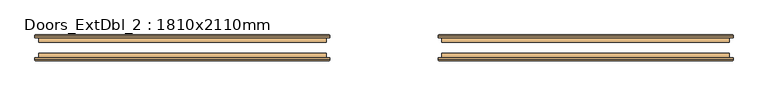
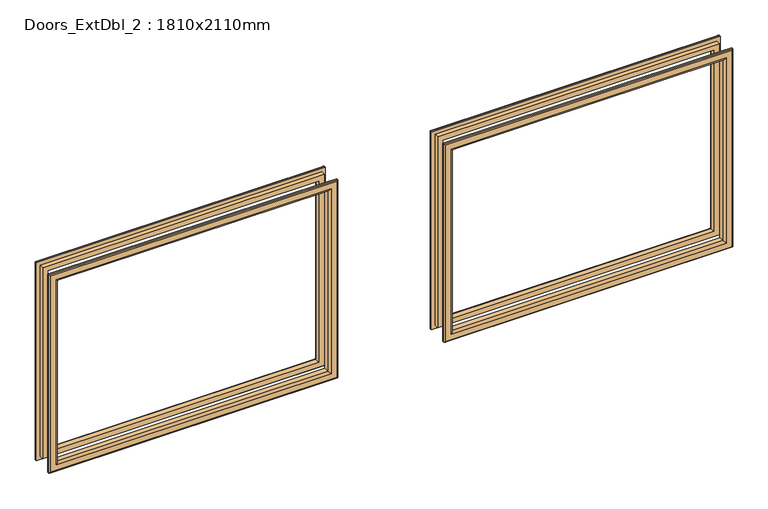
"""IFC4 building model written with IfcOpenShell, lengths in millimetres: door geometry, Doors_ExtDbl_2 : 1810x2110mm."""

from ifc_helpers import new_model, si_unit, frame, origin, place, context, project, spatial, ellipse_curve, source, transform, mapped, element, save
from ifc_brep_helpers import plane_surface, cylinder_surface, advanced_brep


def doors_extdbl_2_1810x2110mm_b7024f51(model_context):
    return source(origin(), model_context, "Body", "AdvancedBrep", [
        advanced_brep(
        [(126.5, 18.4, 808.5), (126.5, 18.4, 358.5), (126.5, 8.4, 358.5), (126.5, 8.4, 808.5), (138.5, 7.4, 796.5), (138.5, 7.4, 370.5), (138.5, 18.4, 370.5), (138.5, 18.4, 796.5), (133.5, 2.4, 801.5), (133.5, 2.4, 365.5), (118.5, 4.4, 816.5), (118.5, 4.4, 350.5), (120.5, 2.4, 352.5), (120.5, 2.4, 814.5), (118.5, 8.4, 816.5), (118.5, 8.4, 350.5), (753.5, 18.4, 358.5), (753.5, 8.4, 358.5), (741.5, 7.4, 370.5), (741.5, 18.4, 370.5), (746.5, 2.4, 365.5), (761.5, 4.4, 350.5), (759.5, 2.4, 352.5), (761.5, 8.4, 350.5), (753.5, 18.4, 808.5), (753.5, 8.4, 808.5), (741.5, 7.4, 796.5), (741.5, 18.4, 796.5), (746.5, 2.4, 801.5), (761.5, 4.4, 816.5), (759.5, 2.4, 814.5), (761.5, 8.4, 816.5)],
        [
            (0, 1),
            (1, 2),
            (2, 3),
            (3, 0),
            (4, 5),
            (5, 6),
            (6, 7),
            (7, 4),
            (8, 9),
            (9, 5, ellipse_curve(frame((133.5, 7.4, 365.5), z_axis=(-0.7071067811865475, 0.0, 0.7071067811865475), x_axis=(0.7071067811865474, 0.0, 0.7071067811865476)), 7.0710678, 5.0)),
            (4, 8, ellipse_curve(frame((133.5, 7.4, 801.5), z_axis=(-0.7071067811865475, 0.0, -0.7071067811865475), x_axis=(-0.7071067811865474, 0.0, 0.7071067811865476)), 7.0710678, 5.0)),
            (10, 11),
            (11, 12, ellipse_curve(frame((120.5, 4.4, 352.5), z_axis=(-0.7071067811865475, 0.0, 0.7071067811865475), x_axis=(0.7071067811865474, 0.0, 0.7071067811865476)), 2.8284271, 2.0)),
            (12, 13),
            (13, 10, ellipse_curve(frame((120.5, 4.4, 814.5), z_axis=(-0.7071067811865475, 0.0, -0.7071067811865475), x_axis=(-0.7071067811865474, 0.0, 0.7071067811865476)), 2.8284271, 2.0)),
            (14, 15),
            (15, 11),
            (10, 14),
            (1, 16),
            (16, 17),
            (17, 2),
            (5, 18),
            (18, 19),
            (19, 6),
            (9, 20),
            (20, 18, ellipse_curve(frame((746.5, 7.4, 365.5), z_axis=(-0.7071067811865475, 0.0, -0.7071067811865475), x_axis=(-0.7071067811865476, 0.0, 0.7071067811865474)), 7.0710678, 5.0)),
            (11, 21),
            (21, 22, ellipse_curve(frame((759.5, 4.4, 352.5), z_axis=(-0.7071067811865475, 0.0, -0.7071067811865475), x_axis=(-0.7071067811865476, 0.0, 0.7071067811865474)), 2.8284271, 2.0)),
            (22, 12),
            (15, 23),
            (23, 21),
            (16, 24),
            (24, 25),
            (25, 17),
            (18, 26),
            (26, 27),
            (27, 19),
            (20, 28),
            (28, 26, ellipse_curve(frame((746.5, 7.4, 801.5), z_axis=(0.7071067811865475, 0.0, -0.7071067811865475), x_axis=(-0.7071067811865474, 0.0, -0.7071067811865476)), 7.0710678, 5.0)),
            (21, 29),
            (29, 30, ellipse_curve(frame((759.5, 4.4, 814.5), z_axis=(0.7071067811865475, 0.0, -0.7071067811865475), x_axis=(-0.7071067811865474, 0.0, -0.7071067811865476)), 2.8284271, 2.0)),
            (30, 22),
            (23, 31),
            (31, 29),
            (14, 31),
            (25, 3),
            (24, 0),
            (27, 7),
            (26, 4),
            (28, 8),
            (30, 13),
            (29, 10),
        ],
        [
            plane_surface(frame((126.5, 8.4, 808.5), z_axis=(-1.0, 0.0, 0.0), x_axis=(0.0, 0.0, -1.0))),
            plane_surface(frame((138.5, 18.4, 796.5), z_axis=(1.0, 0.0, 0.0), x_axis=(0.0, 0.0, -1.0))),
            cylinder_surface(frame((133.5, 7.4, 808.5), z_axis=(0.0, 0.0, 1.0), x_axis=(-1.0, 0.0, 0.0)), 5.0),
            cylinder_surface(frame((120.5, 4.4, 808.5), z_axis=(0.0, 0.0, 1.0), x_axis=(-1.0, 0.0, 0.0)), 2.0),
            plane_surface(frame((118.5, 4.4, 816.5), z_axis=(-1.0, 0.0, 0.0), x_axis=(0.0, 0.0, -1.0))),
            plane_surface(frame((126.5, 8.4, 358.5), z_axis=(0.0, 0.0, -1.0), x_axis=(1.0, 0.0, 0.0))),
            plane_surface(frame((138.5, 18.4, 370.5), z_axis=(0.0, 0.0, 1.0), x_axis=(1.0, 0.0, 0.0))),
            cylinder_surface(frame((126.5, 7.4, 365.5), z_axis=(-1.0, 0.0, 0.0), x_axis=(0.0, 0.0, -1.0)), 5.0),
            cylinder_surface(frame((126.5, 4.4, 352.5), z_axis=(-1.0, 0.0, 0.0), x_axis=(0.0, 0.0, -1.0)), 2.0),
            plane_surface(frame((118.5, 4.4, 350.5), z_axis=(0.0, 0.0, -1.0), x_axis=(1.0, 0.0, 0.0))),
            plane_surface(frame((753.5, 8.4, 358.5), z_axis=(1.0, 0.0, 0.0), x_axis=(0.0, 0.0, 1.0))),
            plane_surface(frame((741.5, 18.4, 370.5), z_axis=(-1.0, 0.0, 0.0), x_axis=(0.0, 0.0, 1.0))),
            cylinder_surface(frame((746.5, 7.4, 358.5), z_axis=(0.0, 0.0, -1.0), x_axis=(1.0, 0.0, 0.0)), 5.0),
            cylinder_surface(frame((759.5, 4.4, 358.5), z_axis=(0.0, 0.0, -1.0), x_axis=(1.0, 0.0, 0.0)), 2.0),
            plane_surface(frame((761.5, 4.4, 350.5), z_axis=(1.0, 0.0, 0.0), x_axis=(0.0, 0.0, 1.0))),
            plane_surface(frame((761.5, 8.4, 816.5), z_axis=(0.0, 1.0, 0.0), x_axis=(-1.0, 0.0, 0.0))),
            plane_surface(frame((753.5, 8.4, 808.5), z_axis=(0.0, 0.0, 1.0), x_axis=(-1.0, 0.0, 0.0))),
            plane_surface(frame((753.5, 18.4, 808.5), z_axis=(0.0, 1.0, 0.0), x_axis=(-1.0, 0.0, 0.0))),
            plane_surface(frame((741.5, 18.4, 796.5), z_axis=(0.0, 0.0, -1.0), x_axis=(-1.0, 0.0, 0.0))),
            cylinder_surface(frame((753.5, 7.4, 801.5), z_axis=(1.0, 0.0, 0.0), x_axis=(0.0, 0.0, 1.0)), 5.0),
            plane_surface(frame((746.5, 2.4, 801.5), z_axis=(0.0, -1.0, 0.0), x_axis=(-1.0, 0.0, 0.0))),
            cylinder_surface(frame((753.5, 4.4, 814.5), z_axis=(1.0, 0.0, 0.0), x_axis=(0.0, 0.0, 1.0)), 2.0),
            plane_surface(frame((761.5, 4.4, 816.5), z_axis=(0.0, 0.0, 1.0), x_axis=(-1.0, 0.0, 0.0))),
        ],
        [
            (0, [[1, 2, 3, 4]]),
            (1, [[5, 6, 7, 8]]),
            (2, [[9, 10, -5, 11]]),
            (3, [[12, 13, 14, 15]]),
            (4, [[16, 17, -12, 18]]),
            (5, [[19, 20, 21, -2]]),
            (6, [[22, 23, 24, -6]]),
            (7, [[25, 26, -22, -10]]),
            (8, [[27, 28, 29, -13]]),
            (9, [[30, 31, -27, -17]]),
            (10, [[32, 33, 34, -20]]),
            (11, [[35, 36, 37, -23]]),
            (12, [[38, 39, -35, -26]]),
            (13, [[40, 41, 42, -28]]),
            (14, [[43, 44, -40, -31]]),
            (15, [[-16, 45, -43, -30], [-3, -21, -34, 46]]),
            (16, [[47, -4, -46, -33]]),
            (17, [[-1, -47, -32, -19], [-7, -24, -37, 48]]),
            (18, [[49, -8, -48, -36]]),
            (19, [[50, -11, -49, -39]]),
            (20, [[-14, -29, -42, 51], [-9, -50, -38, -25]]),
            (21, [[52, -15, -51, -41]]),
            (22, [[-45, -18, -52, -44]]),
        ],
    ),
        advanced_brep(
        [(753.5, 42.4, 808.5), (753.5, 42.4, 358.5), (753.5, 52.4, 358.5), (753.5, 52.4, 808.5), (741.5, 53.4, 796.5), (741.5, 53.4, 370.5), (741.5, 42.4, 370.5), (741.5, 42.4, 796.5), (746.5, 58.4, 801.5), (746.5, 58.4, 365.5), (761.5, 56.4, 816.5), (761.5, 56.4, 350.5), (759.5, 58.4, 352.5), (759.5, 58.4, 814.5), (761.5, 52.4, 816.5), (761.5, 52.4, 350.5), (126.5, 42.4, 358.5), (126.5, 52.4, 358.5), (138.5, 53.4, 370.5), (138.5, 42.4, 370.5), (133.5, 58.4, 365.5), (118.5, 56.4, 350.5), (120.5, 58.4, 352.5), (118.5, 52.4, 350.5), (126.5, 42.4, 808.5), (126.5, 52.4, 808.5), (138.5, 53.4, 796.5), (138.5, 42.4, 796.5), (133.5, 58.4, 801.5), (118.5, 56.4, 816.5), (120.5, 58.4, 814.5), (118.5, 52.4, 816.5)],
        [
            (0, 1),
            (1, 2),
            (2, 3),
            (3, 0),
            (4, 5),
            (5, 6),
            (6, 7),
            (7, 4),
            (8, 9),
            (9, 5, ellipse_curve(frame((746.5, 53.4, 365.5), z_axis=(0.707106781186543, 0.0, 0.707106781186552), x_axis=(-0.707106781186552, 0.0, 0.707106781186543)), 7.0710678, 5.0)),
            (4, 8, ellipse_curve(frame((746.5, 53.4, 801.5), z_axis=(0.7071067811865519, 0.0, -0.707106781186543), x_axis=(0.7071067811865429, 0.0, 0.7071067811865521)), 7.0710678, 5.0)),
            (10, 11),
            (11, 12, ellipse_curve(frame((759.5, 56.4, 352.5), z_axis=(0.707106781186543, 0.0, 0.707106781186552), x_axis=(-0.707106781186552, 0.0, 0.707106781186543)), 2.8284271, 2.0)),
            (12, 13),
            (13, 10, ellipse_curve(frame((759.5, 56.4, 814.5), z_axis=(0.7071067811865519, 0.0, -0.707106781186543), x_axis=(0.7071067811865429, 0.0, 0.7071067811865521)), 2.8284271, 2.0)),
            (14, 15),
            (15, 11),
            (10, 14),
            (1, 16),
            (16, 17),
            (17, 2),
            (5, 18),
            (18, 19),
            (19, 6),
            (9, 20),
            (20, 18, ellipse_curve(frame((133.5, 53.4, 365.5), z_axis=(0.707106781186552, 0.0, -0.7071067811865431), x_axis=(0.7071067811865429, 0.0, 0.7071067811865521)), 7.0710678, 5.0)),
            (11, 21),
            (21, 22, ellipse_curve(frame((120.5, 56.4, 352.5), z_axis=(0.707106781186552, 0.0, -0.7071067811865431), x_axis=(0.7071067811865429, 0.0, 0.7071067811865521)), 2.8284271, 2.0)),
            (22, 12),
            (15, 23),
            (23, 21),
            (16, 24),
            (24, 25),
            (25, 17),
            (18, 26),
            (26, 27),
            (27, 19),
            (20, 28),
            (28, 26, ellipse_curve(frame((133.5, 53.4, 801.5), z_axis=(-0.707106781186543, 0.0, -0.7071067811865519), x_axis=(0.7071067811865517, 0.0, -0.7071067811865432)), 7.0710678, 5.0)),
            (21, 29),
            (29, 30, ellipse_curve(frame((120.5, 56.4, 814.5), z_axis=(-0.707106781186543, 0.0, -0.7071067811865519), x_axis=(0.7071067811865517, 0.0, -0.7071067811865432)), 2.8284271, 2.0)),
            (30, 22),
            (23, 31),
            (31, 29),
            (14, 31),
            (25, 3),
            (24, 0),
            (27, 7),
            (26, 4),
            (28, 8),
            (30, 13),
            (29, 10),
        ],
        [
            plane_surface(frame((753.5, 52.4, 808.5), z_axis=(1.0, 0.0, 0.0), x_axis=(0.0, 0.0, -1.0))),
            plane_surface(frame((741.5, 42.4, 796.5), z_axis=(-1.0, 0.0, 0.0), x_axis=(0.0, 0.0, -1.0))),
            cylinder_surface(frame((746.5, 53.4, 808.5), z_axis=(0.0, 0.0, 1.0), x_axis=(1.0, 0.0, 0.0)), 5.0),
            cylinder_surface(frame((759.5, 56.4, 808.5), z_axis=(0.0, 0.0, 1.0), x_axis=(1.0, 0.0, 0.0)), 2.0),
            plane_surface(frame((761.5, 56.4, 816.5), z_axis=(1.0, 0.0, 0.0), x_axis=(0.0, 0.0, -1.0))),
            plane_surface(frame((753.5, 52.4, 358.5), z_axis=(0.0, 0.0, -1.0), x_axis=(-1.0, 0.0, 0.0))),
            plane_surface(frame((741.5, 42.4, 370.5), z_axis=(0.0, 0.0, 1.0), x_axis=(-1.0, 0.0, 0.0))),
            cylinder_surface(frame((753.5, 53.4, 365.5), z_axis=(1.0, 0.0, 0.0), x_axis=(0.0, 0.0, -1.0)), 5.0),
            cylinder_surface(frame((753.5, 56.4, 352.5), z_axis=(1.0, 0.0, 0.0), x_axis=(0.0, 0.0, -1.0)), 2.0),
            plane_surface(frame((761.5, 56.4, 350.5), z_axis=(0.0, 0.0, -1.0), x_axis=(-1.0, 0.0, 0.0))),
            plane_surface(frame((126.5, 52.4, 358.5), z_axis=(-1.0, 0.0, 0.0), x_axis=(0.0, 0.0, 1.0))),
            plane_surface(frame((138.5, 42.4, 370.5), z_axis=(1.0, 0.0, 0.0), x_axis=(0.0, 0.0, 1.0))),
            cylinder_surface(frame((133.5, 53.4, 358.5), z_axis=(0.0, 0.0, -1.0), x_axis=(-1.0, 0.0, 0.0)), 5.0),
            cylinder_surface(frame((120.5, 56.4, 358.5), z_axis=(0.0, 0.0, -1.0), x_axis=(-1.0, 0.0, 0.0)), 2.0),
            plane_surface(frame((118.5, 56.4, 350.5), z_axis=(-1.0, 0.0, 0.0), x_axis=(0.0, 0.0, 1.0))),
            plane_surface(frame((118.5, 52.4, 816.5), z_axis=(0.0, -1.0, 0.0), x_axis=(1.0, 0.0, 0.0))),
            plane_surface(frame((126.5, 52.4, 808.5), z_axis=(0.0, 0.0, 1.0), x_axis=(1.0, 0.0, 0.0))),
            plane_surface(frame((126.5, 42.4, 808.5), z_axis=(0.0, -1.0, 0.0), x_axis=(1.0, 0.0, 0.0))),
            plane_surface(frame((138.5, 42.4, 796.5), z_axis=(0.0, 0.0, -1.0), x_axis=(1.0, 0.0, 0.0))),
            cylinder_surface(frame((126.5, 53.4, 801.5), z_axis=(-1.0, 0.0, 0.0), x_axis=(0.0, 0.0, 1.0)), 5.0),
            plane_surface(frame((133.5, 58.4, 801.5), z_axis=(0.0, 1.0, 0.0), x_axis=(1.0, 0.0, 0.0))),
            cylinder_surface(frame((126.5, 56.4, 814.5), z_axis=(-1.0, 0.0, 0.0), x_axis=(0.0, 0.0, 1.0)), 2.0),
            plane_surface(frame((118.5, 56.4, 816.5), z_axis=(0.0, 0.0, 1.0), x_axis=(1.0, 0.0, 0.0))),
        ],
        [
            (0, [[1, 2, 3, 4]]),
            (1, [[5, 6, 7, 8]]),
            (2, [[9, 10, -5, 11]]),
            (3, [[12, 13, 14, 15]]),
            (4, [[16, 17, -12, 18]]),
            (5, [[19, 20, 21, -2]]),
            (6, [[22, 23, 24, -6]]),
            (7, [[25, 26, -22, -10]]),
            (8, [[27, 28, 29, -13]]),
            (9, [[30, 31, -27, -17]]),
            (10, [[32, 33, 34, -20]]),
            (11, [[35, 36, 37, -23]]),
            (12, [[38, 39, -35, -26]]),
            (13, [[40, 41, 42, -28]]),
            (14, [[43, 44, -40, -31]]),
            (15, [[-16, 45, -43, -30], [-3, -21, -34, 46]]),
            (16, [[47, -4, -46, -33]]),
            (17, [[-1, -47, -32, -19], [-7, -24, -37, 48]]),
            (18, [[49, -8, -48, -36]]),
            (19, [[50, -11, -49, -39]]),
            (20, [[-14, -29, -42, 51], [-9, -50, -38, -25]]),
            (21, [[52, -15, -51, -41]]),
            (22, [[-45, -18, -52, -44]]),
        ],
    ),
        advanced_brep(
        [(-753.5, 18.4, 808.5), (-753.5, 18.4, 358.5), (-753.5, 8.4, 358.5), (-753.5, 8.4, 808.5), (-741.5, 7.4, 796.5), (-741.5, 7.4, 370.5), (-741.5, 18.4, 370.5), (-741.5, 18.4, 796.5), (-746.5, 2.4, 801.5), (-746.5, 2.4, 365.5), (-761.5, 4.4, 816.5), (-761.5, 4.4, 350.5), (-759.5, 2.4, 352.5), (-759.5, 2.4, 814.5), (-761.5, 8.4, 816.5), (-761.5, 8.4, 350.5), (-126.5, 18.4, 358.5), (-126.5, 8.4, 358.5), (-138.5, 7.4, 370.5), (-138.5, 18.4, 370.5), (-133.5, 2.4, 365.5), (-118.5, 4.4, 350.5), (-120.5, 2.4, 352.5), (-118.5, 8.4, 350.5), (-126.5, 18.4, 808.5), (-126.5, 8.4, 808.5), (-138.5, 7.4, 796.5), (-138.5, 18.4, 796.5), (-133.5, 2.4, 801.5), (-118.5, 4.4, 816.5), (-120.5, 2.4, 814.5), (-118.5, 8.4, 816.5)],
        [
            (0, 1),
            (1, 2),
            (2, 3),
            (3, 0),
            (4, 5),
            (5, 6),
            (6, 7),
            (7, 4),
            (8, 9),
            (9, 5, ellipse_curve(frame((-746.5, 7.4, 365.5), z_axis=(-0.7071067811865475, 0.0, 0.7071067811865475), x_axis=(0.7071067811865474, 0.0, 0.7071067811865476)), 7.0710678, 5.0)),
            (4, 8, ellipse_curve(frame((-746.5, 7.4, 801.5), z_axis=(-0.7071067811865476, 0.0, -0.7071067811865475), x_axis=(-0.7071067811865475, 0.0, 0.7071067811865476)), 7.0710678, 5.0)),
            (10, 11),
            (11, 12, ellipse_curve(frame((-759.5, 4.4, 352.5), z_axis=(-0.7071067811865475, 0.0, 0.7071067811865475), x_axis=(0.7071067811865474, 0.0, 0.7071067811865476)), 2.8284271, 2.0)),
            (12, 13),
            (13, 10, ellipse_curve(frame((-759.5, 4.4, 814.5), z_axis=(-0.7071067811865476, 0.0, -0.7071067811865475), x_axis=(-0.7071067811865475, 0.0, 0.7071067811865476)), 2.8284271, 2.0)),
            (14, 15),
            (15, 11),
            (10, 14),
            (1, 16),
            (16, 17),
            (17, 2),
            (5, 18),
            (18, 19),
            (19, 6),
            (9, 20),
            (20, 18, ellipse_curve(frame((-133.5, 7.4, 365.5), z_axis=(-0.7071067811865475, 0.0, -0.7071067811865475), x_axis=(-0.7071067811865476, 0.0, 0.7071067811865474)), 7.0710678, 5.0)),
            (11, 21),
            (21, 22, ellipse_curve(frame((-120.5, 4.4, 352.5), z_axis=(-0.7071067811865475, 0.0, -0.7071067811865475), x_axis=(-0.7071067811865476, 0.0, 0.7071067811865474)), 2.8284271, 2.0)),
            (22, 12),
            (15, 23),
            (23, 21),
            (16, 24),
            (24, 25),
            (25, 17),
            (18, 26),
            (26, 27),
            (27, 19),
            (20, 28),
            (28, 26, ellipse_curve(frame((-133.5, 7.4, 801.5), z_axis=(0.7071067811865475, 0.0, -0.7071067811865476), x_axis=(-0.7071067811865476, 0.0, -0.7071067811865475)), 7.0710678, 5.0)),
            (21, 29),
            (29, 30, ellipse_curve(frame((-120.5, 4.4, 814.5), z_axis=(0.7071067811865475, 0.0, -0.7071067811865476), x_axis=(-0.7071067811865476, 0.0, -0.7071067811865475)), 2.8284271, 2.0)),
            (30, 22),
            (23, 31),
            (31, 29),
            (14, 31),
            (25, 3),
            (24, 0),
            (27, 7),
            (26, 4),
            (28, 8),
            (30, 13),
            (29, 10),
        ],
        [
            plane_surface(frame((-753.5, 8.4, 808.5), z_axis=(-1.0, 0.0, 0.0), x_axis=(0.0, 0.0, -1.0))),
            plane_surface(frame((-741.5, 18.4, 796.5), z_axis=(1.0, 0.0, 0.0), x_axis=(0.0, 0.0, -1.0))),
            cylinder_surface(frame((-746.5, 7.4, 808.5), z_axis=(0.0, 0.0, 1.0), x_axis=(-1.0, 0.0, 0.0)), 5.0),
            cylinder_surface(frame((-759.5, 4.4, 808.5), z_axis=(0.0, 0.0, 1.0), x_axis=(-1.0, 0.0, 0.0)), 2.0),
            plane_surface(frame((-761.5, 4.4, 816.5), z_axis=(-1.0, 0.0, 0.0), x_axis=(0.0, 0.0, -1.0))),
            plane_surface(frame((-753.5, 8.4, 358.5), z_axis=(0.0, 0.0, -1.0), x_axis=(1.0, 0.0, 0.0))),
            plane_surface(frame((-741.5, 18.4, 370.5), z_axis=(0.0, 0.0, 1.0), x_axis=(1.0, 0.0, 0.0))),
            cylinder_surface(frame((-753.5, 7.4, 365.5), z_axis=(-1.0, 0.0, 0.0), x_axis=(0.0, 0.0, -1.0)), 5.0),
            cylinder_surface(frame((-753.5, 4.4, 352.5), z_axis=(-1.0, 0.0, 0.0), x_axis=(0.0, 0.0, -1.0)), 2.0),
            plane_surface(frame((-761.5, 4.4, 350.5), z_axis=(0.0, 0.0, -1.0), x_axis=(1.0, 0.0, 0.0))),
            plane_surface(frame((-126.5, 8.4, 358.5), z_axis=(1.0, 0.0, 0.0), x_axis=(0.0, 0.0, 1.0))),
            plane_surface(frame((-138.5, 18.4, 370.5), z_axis=(-1.0, 0.0, 0.0), x_axis=(0.0, 0.0, 1.0))),
            cylinder_surface(frame((-133.5, 7.4, 358.5), z_axis=(0.0, 0.0, -1.0), x_axis=(1.0, 0.0, 0.0)), 5.0),
            cylinder_surface(frame((-120.5, 4.4, 358.5), z_axis=(0.0, 0.0, -1.0), x_axis=(1.0, 0.0, 0.0)), 2.0),
            plane_surface(frame((-118.5, 4.4, 350.5), z_axis=(1.0, 0.0, 0.0), x_axis=(0.0, 0.0, 1.0))),
            plane_surface(frame((-118.5, 8.4, 816.5), z_axis=(0.0, 1.0, 0.0), x_axis=(-1.0, 0.0, 0.0))),
            plane_surface(frame((-126.5, 8.4, 808.5), z_axis=(0.0, 0.0, 1.0), x_axis=(-1.0, 0.0, 0.0))),
            plane_surface(frame((-126.5, 18.4, 808.5), z_axis=(0.0, 1.0, 0.0), x_axis=(-1.0, 0.0, 0.0))),
            plane_surface(frame((-138.5, 18.4, 796.5), z_axis=(0.0, 0.0, -1.0), x_axis=(-1.0, 0.0, 0.0))),
            cylinder_surface(frame((-126.5, 7.4, 801.5), z_axis=(1.0, 0.0, 0.0), x_axis=(0.0, 0.0, 1.0)), 5.0),
            plane_surface(frame((-133.5, 2.4, 801.5), z_axis=(0.0, -1.0, 0.0), x_axis=(-1.0, 0.0, 0.0))),
            cylinder_surface(frame((-126.5, 4.4, 814.5), z_axis=(1.0, 0.0, 0.0), x_axis=(0.0, 0.0, 1.0)), 2.0),
            plane_surface(frame((-118.5, 4.4, 816.5), z_axis=(0.0, 0.0, 1.0), x_axis=(-1.0, 0.0, 0.0))),
        ],
        [
            (0, [[1, 2, 3, 4]]),
            (1, [[5, 6, 7, 8]]),
            (2, [[9, 10, -5, 11]]),
            (3, [[12, 13, 14, 15]]),
            (4, [[16, 17, -12, 18]]),
            (5, [[19, 20, 21, -2]]),
            (6, [[22, 23, 24, -6]]),
            (7, [[25, 26, -22, -10]]),
            (8, [[27, 28, 29, -13]]),
            (9, [[30, 31, -27, -17]]),
            (10, [[32, 33, 34, -20]]),
            (11, [[35, 36, 37, -23]]),
            (12, [[38, 39, -35, -26]]),
            (13, [[40, 41, 42, -28]]),
            (14, [[43, 44, -40, -31]]),
            (15, [[-16, 45, -43, -30], [-3, -21, -34, 46]]),
            (16, [[47, -4, -46, -33]]),
            (17, [[-1, -47, -32, -19], [-7, -24, -37, 48]]),
            (18, [[49, -8, -48, -36]]),
            (19, [[50, -11, -49, -39]]),
            (20, [[-14, -29, -42, 51], [-9, -50, -38, -25]]),
            (21, [[52, -15, -51, -41]]),
            (22, [[-45, -18, -52, -44]]),
        ],
    ),
        advanced_brep(
        [(-126.5, 42.4, 808.5), (-126.5, 42.4, 358.5), (-126.5, 52.4, 358.5), (-126.5, 52.4, 808.5), (-138.5, 53.4, 796.5), (-138.5, 53.4, 370.5), (-138.5, 42.4, 370.5), (-138.5, 42.4, 796.5), (-133.5, 58.4, 801.5), (-133.5, 58.4, 365.5), (-118.5, 56.4, 816.5), (-118.5, 56.4, 350.5), (-120.5, 58.4, 352.5), (-120.5, 58.4, 814.5), (-118.5, 52.4, 816.5), (-118.5, 52.4, 350.5), (-753.5, 42.4, 358.5), (-753.5, 52.4, 358.5), (-741.5, 53.4, 370.5), (-741.5, 42.4, 370.5), (-746.5, 58.4, 365.5), (-761.5, 56.4, 350.5), (-759.5, 58.4, 352.5), (-761.5, 52.4, 350.5), (-753.5, 42.4, 808.5), (-753.5, 52.4, 808.5), (-741.5, 53.4, 796.5), (-741.5, 42.4, 796.5), (-746.5, 58.4, 801.5), (-761.5, 56.4, 816.5), (-759.5, 58.4, 814.5), (-761.5, 52.4, 816.5)],
        [
            (0, 1),
            (1, 2),
            (2, 3),
            (3, 0),
            (4, 5),
            (5, 6),
            (6, 7),
            (7, 4),
            (8, 9),
            (9, 5, ellipse_curve(frame((-133.5, 53.4, 365.5), z_axis=(0.707106781186543, 0.0, 0.707106781186552), x_axis=(-0.707106781186552, 0.0, 0.707106781186543)), 7.0710678, 5.0)),
            (4, 8, ellipse_curve(frame((-133.5, 53.4, 801.5), z_axis=(0.707106781186552, 0.0, -0.707106781186543), x_axis=(0.7071067811865429, 0.0, 0.707106781186552)), 7.0710678, 5.0)),
            (10, 11),
            (11, 12, ellipse_curve(frame((-120.5, 56.4, 352.5), z_axis=(0.707106781186543, 0.0, 0.707106781186552), x_axis=(-0.707106781186552, 0.0, 0.707106781186543)), 2.8284271, 2.0)),
            (12, 13),
            (13, 10, ellipse_curve(frame((-120.5, 56.4, 814.5), z_axis=(0.707106781186552, 0.0, -0.707106781186543), x_axis=(0.7071067811865429, 0.0, 0.707106781186552)), 2.8284271, 2.0)),
            (14, 15),
            (15, 11),
            (10, 14),
            (1, 16),
            (16, 17),
            (17, 2),
            (5, 18),
            (18, 19),
            (19, 6),
            (9, 20),
            (20, 18, ellipse_curve(frame((-746.5, 53.4, 365.5), z_axis=(0.707106781186552, 0.0, -0.707106781186543), x_axis=(0.7071067811865429, 0.0, 0.707106781186552)), 7.0710678, 5.0)),
            (11, 21),
            (21, 22, ellipse_curve(frame((-759.5, 56.4, 352.5), z_axis=(0.707106781186552, 0.0, -0.707106781186543), x_axis=(0.7071067811865429, 0.0, 0.707106781186552)), 2.8284271, 2.0)),
            (22, 12),
            (15, 23),
            (23, 21),
            (16, 24),
            (24, 25),
            (25, 17),
            (18, 26),
            (26, 27),
            (27, 19),
            (20, 28),
            (28, 26, ellipse_curve(frame((-746.5, 53.4, 801.5), z_axis=(-0.7071067811865429, 0.0, -0.707106781186552), x_axis=(0.7071067811865519, 0.0, -0.707106781186543)), 7.0710678, 5.0)),
            (21, 29),
            (29, 30, ellipse_curve(frame((-759.5, 56.4, 814.5), z_axis=(-0.7071067811865429, 0.0, -0.707106781186552), x_axis=(0.7071067811865519, 0.0, -0.707106781186543)), 2.8284271, 2.0)),
            (30, 22),
            (23, 31),
            (31, 29),
            (14, 31),
            (25, 3),
            (24, 0),
            (27, 7),
            (26, 4),
            (28, 8),
            (30, 13),
            (29, 10),
        ],
        [
            plane_surface(frame((-126.5, 52.4, 808.5), z_axis=(1.0, 0.0, 0.0), x_axis=(0.0, 0.0, -1.0))),
            plane_surface(frame((-138.5, 42.4, 796.5), z_axis=(-1.0, 0.0, 0.0), x_axis=(0.0, 0.0, -1.0))),
            cylinder_surface(frame((-133.5, 53.4, 808.5), z_axis=(0.0, 0.0, 1.0), x_axis=(1.0, 0.0, 0.0)), 5.0),
            cylinder_surface(frame((-120.5, 56.4, 808.5), z_axis=(0.0, 0.0, 1.0), x_axis=(1.0, 0.0, 0.0)), 2.0),
            plane_surface(frame((-118.5, 56.4, 816.5), z_axis=(1.0, 0.0, 0.0), x_axis=(0.0, 0.0, -1.0))),
            plane_surface(frame((-126.5, 52.4, 358.5), z_axis=(0.0, 0.0, -1.0), x_axis=(-1.0, 0.0, 0.0))),
            plane_surface(frame((-138.5, 42.4, 370.5), z_axis=(0.0, 0.0, 1.0), x_axis=(-1.0, 0.0, 0.0))),
            cylinder_surface(frame((-126.5, 53.4, 365.5), z_axis=(1.0, 0.0, 0.0), x_axis=(0.0, 0.0, -1.0)), 5.0),
            cylinder_surface(frame((-126.5, 56.4, 352.5), z_axis=(1.0, 0.0, 0.0), x_axis=(0.0, 0.0, -1.0)), 2.0),
            plane_surface(frame((-118.5, 56.4, 350.5), z_axis=(0.0, 0.0, -1.0), x_axis=(-1.0, 0.0, 0.0))),
            plane_surface(frame((-753.5, 52.4, 358.5), z_axis=(-1.0, 0.0, 0.0), x_axis=(0.0, 0.0, 1.0))),
            plane_surface(frame((-741.5, 42.4, 370.5), z_axis=(1.0, 0.0, 0.0), x_axis=(0.0, 0.0, 1.0))),
            cylinder_surface(frame((-746.5, 53.4, 358.5), z_axis=(0.0, 0.0, -1.0), x_axis=(-1.0, 0.0, 0.0)), 5.0),
            cylinder_surface(frame((-759.5, 56.4, 358.5), z_axis=(0.0, 0.0, -1.0), x_axis=(-1.0, 0.0, 0.0)), 2.0),
            plane_surface(frame((-761.5, 56.4, 350.5), z_axis=(-1.0, 0.0, 0.0), x_axis=(0.0, 0.0, 1.0))),
            plane_surface(frame((-761.5, 52.4, 816.5), z_axis=(0.0, -1.0, 0.0), x_axis=(1.0, 0.0, 0.0))),
            plane_surface(frame((-753.5, 52.4, 808.5), z_axis=(0.0, 0.0, 1.0), x_axis=(1.0, 0.0, 0.0))),
            plane_surface(frame((-753.5, 42.4, 808.5), z_axis=(0.0, -1.0, 0.0), x_axis=(1.0, 0.0, 0.0))),
            plane_surface(frame((-741.5, 42.4, 796.5), z_axis=(0.0, 0.0, -1.0), x_axis=(1.0, 0.0, 0.0))),
            cylinder_surface(frame((-753.5, 53.4, 801.5), z_axis=(-1.0, 0.0, 0.0), x_axis=(0.0, 0.0, 1.0)), 5.0),
            plane_surface(frame((-746.5, 58.4, 801.5), z_axis=(0.0, 1.0, 0.0), x_axis=(1.0, 0.0, 0.0))),
            cylinder_surface(frame((-753.5, 56.4, 814.5), z_axis=(-1.0, 0.0, 0.0), x_axis=(0.0, 0.0, 1.0)), 2.0),
            plane_surface(frame((-761.5, 56.4, 816.5), z_axis=(0.0, 0.0, 1.0), x_axis=(1.0, 0.0, 0.0))),
        ],
        [
            (0, [[1, 2, 3, 4]]),
            (1, [[5, 6, 7, 8]]),
            (2, [[9, 10, -5, 11]]),
            (3, [[12, 13, 14, 15]]),
            (4, [[16, 17, -12, 18]]),
            (5, [[19, 20, 21, -2]]),
            (6, [[22, 23, 24, -6]]),
            (7, [[25, 26, -22, -10]]),
            (8, [[27, 28, 29, -13]]),
            (9, [[30, 31, -27, -17]]),
            (10, [[32, 33, 34, -20]]),
            (11, [[35, 36, 37, -23]]),
            (12, [[38, 39, -35, -26]]),
            (13, [[40, 41, 42, -28]]),
            (14, [[43, 44, -40, -31]]),
            (15, [[-16, 45, -43, -30], [-3, -21, -34, 46]]),
            (16, [[47, -4, -46, -33]]),
            (17, [[-1, -47, -32, -19], [-7, -24, -37, 48]]),
            (18, [[49, -8, -48, -36]]),
            (19, [[50, -11, -49, -39]]),
            (20, [[-14, -29, -42, 51], [-9, -50, -38, -25]]),
            (21, [[52, -15, -51, -41]]),
            (22, [[-45, -18, -52, -44]]),
        ],
    ),
    ])


if __name__ == "__main__":
    model = new_model("IFC4")
    model_context = context("Model", 3, world=origin())
    ifc_project = project(units=[si_unit("LENGTHUNIT", "METRE", prefix="MILLI")], contexts=[model_context])
    site = spatial("IfcSite", under=ifc_project)
    building = spatial("IfcBuilding", under=site)
    placement = place(None, origin())
    doors_extdbl_2_1810x2110mm_shape = doors_extdbl_2_1810x2110mm_b7024f51(model_context)
    element("IfcDoor", 1, ObjectType="Doors_ExtDbl_2 : 1810x2110mm", at=placement, inside=building, context=model_context, shape_type="MappedRepresentation", body=[
        mapped(doors_extdbl_2_1810x2110mm_shape, transform((0.0, 0.0, 0.0), x_axis=(1.0, 0.0, 0.0), y_axis=(0.0, 1.0, 0.0), z_axis=(0.0, 0.0, 1.0))),
    ])
    save(model, "model.ifc")

# Revit data of these elements
# Type "Doors_ExtDbl_2 : 1810x2110mm"
#   Type Mark = "8"
#   Type Comments = "External Double"
#   Operation = "DoubleDoorSingleSwing"
#   Construction Type Id = "GSP4R"
#   Keynote = "L20"
#   Analytic Construction = "1/8 in Pilkington single glazing"
#   Wrap Layers (Int) from Ext = 0' - 6.98819"
#   Wrap Layers (Ext) from Ext = 0' - 4.03543"
#   Visual Light Transmittance = 0.9
#   Top of Lock Rail = 2' - 11.43307"
#   Thickness = 0' - 1.73228"
#   Stile Shutting = 0' - 4.92126"
#   Stile - Top Rail = 0' - 5.90551"
#   Stile - Lock Rail = 0' - 5.90551"
#   Stile - Hanging = 0' - 3.93701"
#   Stile - Bottom Rail = 0' - 11.81102"
#   Solar Heat Gain Coefficient = 0.78
#   Rough Width = 5' - 11.25984"
#   Rough Height = 6' - 11.07087"
#   O/A Frame Width = 0' - 2.51969"
#   Heat Transfer Coefficient (U) = 0.6496 BTU/(h·ft²·°F)
#   Handle Z Distance = 3' - 1.40157"
#   Glazing Thickness = 0' - 0.94488"
#   FrameWidth = 0' - 1.65354"
#   FrameOffset - External = 0' - 2.55906"
#   FrameDepth = 0' - 3.50394"
#   Door Panel Width = 2' - 9.54331"
#   Door Panel Thickness = 0' - 1.73228"
#   Door Panel Height = 6' - 6.74016"
#   Cill Thickness = 0' - 2.14567"
#   Cill Projection = 0' - 1.1811"
#   Handle X Distance = 0' - 2.95276"
#   Height = 6' - 11.07087"
#   Structural Tolerance = 0' - 0.25591"
#   Tolerance = 0' - 0.11811"
#   Undercut = 0' - 0.15748"
#   Width = 5' - 11.25984"
#   Cill Extension = 0' - 0.98425"
#   Cavity Closer Width = 0' - 1.9685"
#   Cavity Closer Offset from Ext = 0' - 4.03543"
#   Cavity Closer Depth = 0' - 3.34646"
#   Vis - Ironmongery = yes
#   Vis - Cavity Closers = yes
#   Define Thermal Properties by = 1
#   Function = 1
#   Material Glass = Door - Glazing
#   Handle Style = element 387460
#   Material Door = Door - Panel
#   Material Frame = Door - Frame/Mullion
#   Material Ironmongery = Door - Handle
#   Wall Closure = (empty or 0)
# Element 1 (IfcDoor, "Doors_ExtDbl_2 : 1810x2110mm")
#   Materials on its faces: "Door - Panel", "Door - Handle", "Door - Frame/Mullion", "Door - Glazing"
# Materials
#   "Door - Glazing": colour RGB 0 0 255, transparency 0.75
#   "Door - Panel": class "Wood", colour RGB 210 159 95, transparency 0, Cost = 0
#   "Door - Frame/Mullion": class "Wood", colour RGB 212 179 113, transparency 0
#   "Door - Handle": colour RGB 247 247 247, transparency 0
